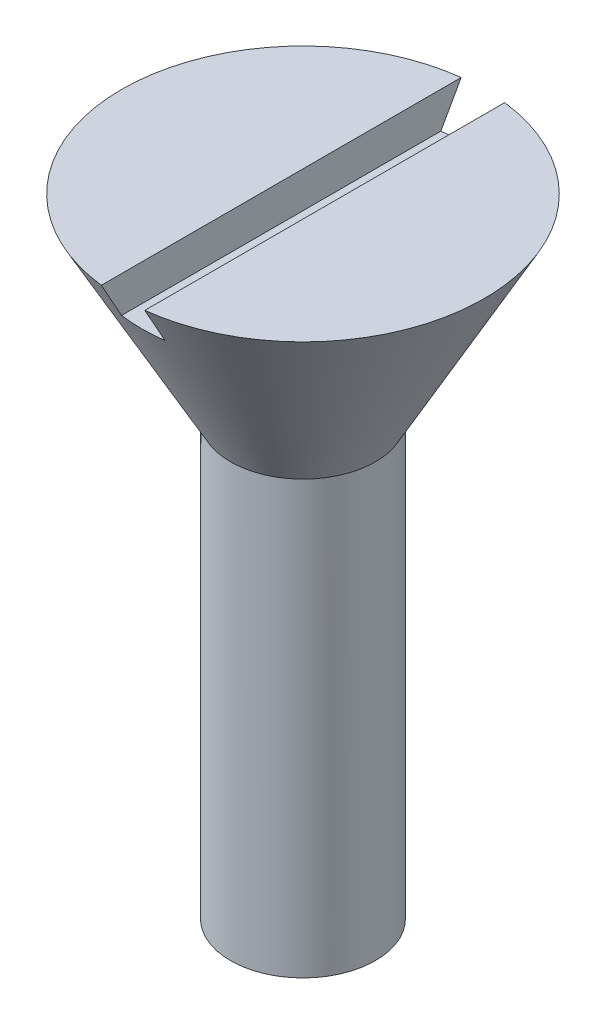
from build123d import *

# Parameters (mm, degrees)
HEAD_SLOT_CUT_DEPTH      = 72.232015274
HEAD_SLOT_CUT_DEPTH_BACK = 72.232015274
HEAD_SLOT_SKETCH_W       = 3
HEAD_SLOT_SKETCH_H       = 7
TRIM_CUT_1_DEPTH         = 72.216220063
TRIM_CUT_1_DEPTH_BACK    = 72.216220063
TRIM_CUT_1_SKETCH_W      = 30.281079354
TRIM_CUT_1_SKETCH_H      = 4.498315547
TRIM_CUT_2_DEPTH         = 66.899626103
TRIM_CUT_2_DEPTH_BACK    = 66.899626103
TRIM_CUT_2_SKETCH_W      = 29.08434912
TRIM_CUT_2_SKETCH_H      = 20.204065749


with BuildPart() as part:
    # Screw Half Profile Sketch → Screw Body Revolve (revolve)
    with BuildSketch(Plane.XY, mode=Mode.PRIVATE) as screw_body_revolve_sk:
        Polygon((0, 0), (5, 0), (5, 50), (15, 68), (0, 68), align=None)
    revolve(screw_body_revolve_sk.sketch.rotate(Axis((0, 68, 0), (0, -1, 0)), 180), axis=Axis((0, 68, 0), (0, -1, 0)))

    # Head Slot Sketch → Head Slot Cut (cut, two sides: drawn at the far end of the back side and taken through both)
    with BuildSketch(Plane.XY.offset(-HEAD_SLOT_CUT_DEPTH_BACK)):
        with Locations((0, 64.5)):
            Rectangle(HEAD_SLOT_SKETCH_W, HEAD_SLOT_SKETCH_H)
    extrude(amount=HEAD_SLOT_CUT_DEPTH + HEAD_SLOT_CUT_DEPTH_BACK, mode=Mode.SUBTRACT)

    # Trim Cut 1 Sketch → Trim Cut 1 (cut, two sides: drawn at the far end of the back side and taken through both)
    with BuildSketch(Plane.XY.offset(-TRIM_CUT_1_DEPTH_BACK)):
        with Locations((0.140539677, 65.750842226)):
            Rectangle(TRIM_CUT_1_SKETCH_W, TRIM_CUT_1_SKETCH_H)
    extrude(amount=TRIM_CUT_1_DEPTH + TRIM_CUT_1_DEPTH_BACK, mode=Mode.SUBTRACT)

    # Trim Cut 2 Sketch → Trim Cut 2 (cut, two sides: drawn at the far end of the back side and taken through both)
    with BuildSketch(Plane.XY.offset(-TRIM_CUT_2_DEPTH_BACK)):
        with Locations((-3.623465422, 10.102032875)):
            Rectangle(TRIM_CUT_2_SKETCH_W, TRIM_CUT_2_SKETCH_H)
    extrude(amount=TRIM_CUT_2_DEPTH + TRIM_CUT_2_DEPTH_BACK, mode=Mode.SUBTRACT)


solid = part.part
